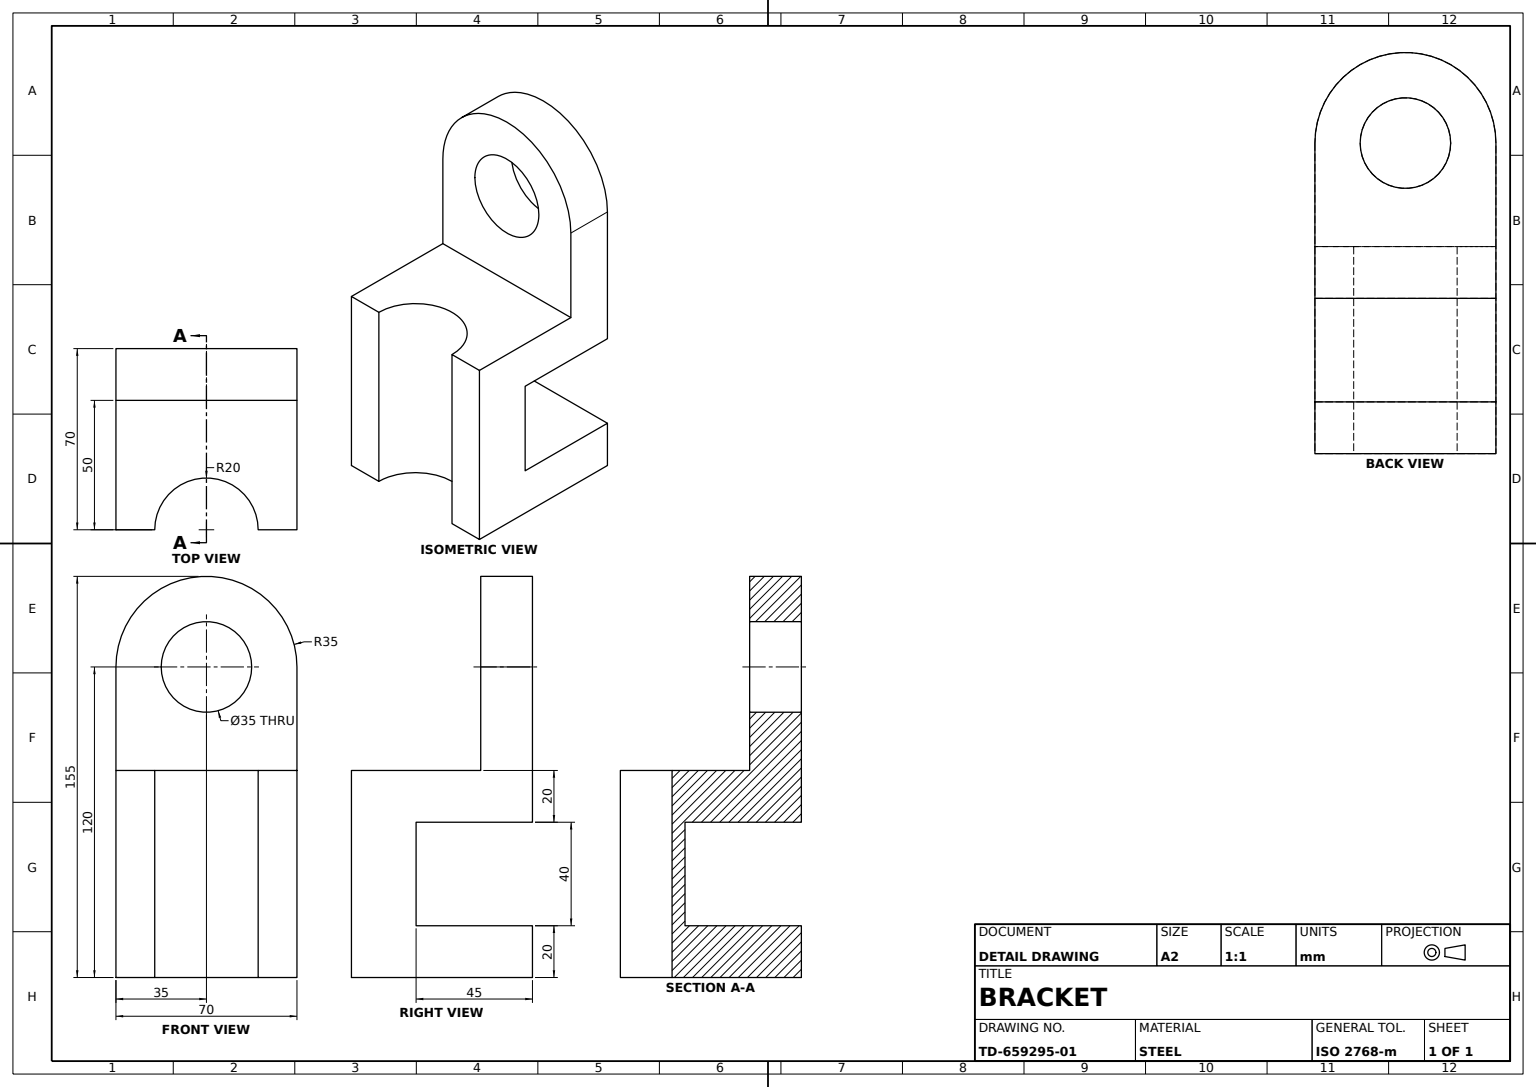
from build123d import *

# Parameters (mm, degrees)
BASE_BLOCK_DEPTH        = 20
BODY_PROFILE_W          = 70
BODY_PROFILE_H          = 25
BODY_SECTION_DEPTH      = 40
SHELF_PROFILE_W         = 70
SHELF_PROFILE_H         = 70
SHELF_BLOCK_DEPTH       = 20
UPRIGHT_PROFILE_W       = 70
UPRIGHT_PROFILE_H       = 20
UPRIGHT_WALL_DEPTH      = 40
ROUNDED_LUG_DEPTH       = 20
LUG_HOLE_PROFILE_R      = 17.5
LUG_THROUGH_HOLE_DEPTH  = 208
HALF_BEARING_BORE_DEPTH = 208


with BuildPart() as part:
    # Base Profile → Base Block (new body)
    with BuildSketch(Plane(origin=(0, 0, 0), x_dir=(1, 0, 0), z_dir=(0, 1, 0))):
        Polygon((35, 0), (35, 35), (-35, 35), (-35, -35), (35, -35), align=None)
    extrude(amount=BASE_BLOCK_DEPTH)

    # Body Profile → Body Section (add)
    with BuildSketch(Plane(origin=(0, 20, 0), x_dir=(1, 0, 0), z_dir=(0, 1, 0))):
        with Locations((0, -22.5)):
            Rectangle(BODY_PROFILE_W, BODY_PROFILE_H)
    extrude(amount=BODY_SECTION_DEPTH)

    # Shelf Profile → Shelf Block (add)
    with BuildSketch(Plane(origin=(0, 60, 0), x_dir=(1, 0, 0), z_dir=(0, 1, 0))):
        Rectangle(SHELF_PROFILE_W, SHELF_PROFILE_H)
    extrude(amount=SHELF_BLOCK_DEPTH)

    # Upright Profile → Upright Wall (add)
    with BuildSketch(Plane(origin=(0, 80, 0), x_dir=(1, 0, 0), z_dir=(0, 1, 0))):
        with Locations((0, 25)):
            Rectangle(UPRIGHT_PROFILE_W, UPRIGHT_PROFILE_H)
    extrude(amount=UPRIGHT_WALL_DEPTH)

    # Lug Profile → Rounded Lug (add)
    with BuildSketch(Plane.XY.offset(-15)):
        with BuildLine():
            Line((-35, 120), (35, 120))
            ThreePointArc((35, 120), (0, 155), (-35, 120))
        make_face()
    extrude(amount=-ROUNDED_LUG_DEPTH)

    # Lug Hole Profile → Lug Through Hole (cut)
    with BuildSketch(Plane.XY.offset(-15)):
        with Locations((0, 120)):
            Circle(LUG_HOLE_PROFILE_R)
    extrude(amount=-LUG_THROUGH_HOLE_DEPTH, mode=Mode.SUBTRACT)

    # Bearing Bore Profile → Half Bearing Bore (cut)
    with BuildSketch(Plane(origin=(0, 80, 0), x_dir=(1, 0, 0), z_dir=(0, 1, 0))):
        with BuildLine():
            Line((-20, -35), (20, -35))
            ThreePointArc((20, -35), (0, -15), (-20, -35))
        make_face()
    extrude(amount=-HALF_BEARING_BORE_DEPTH, mode=Mode.SUBTRACT)


solid = part.part
